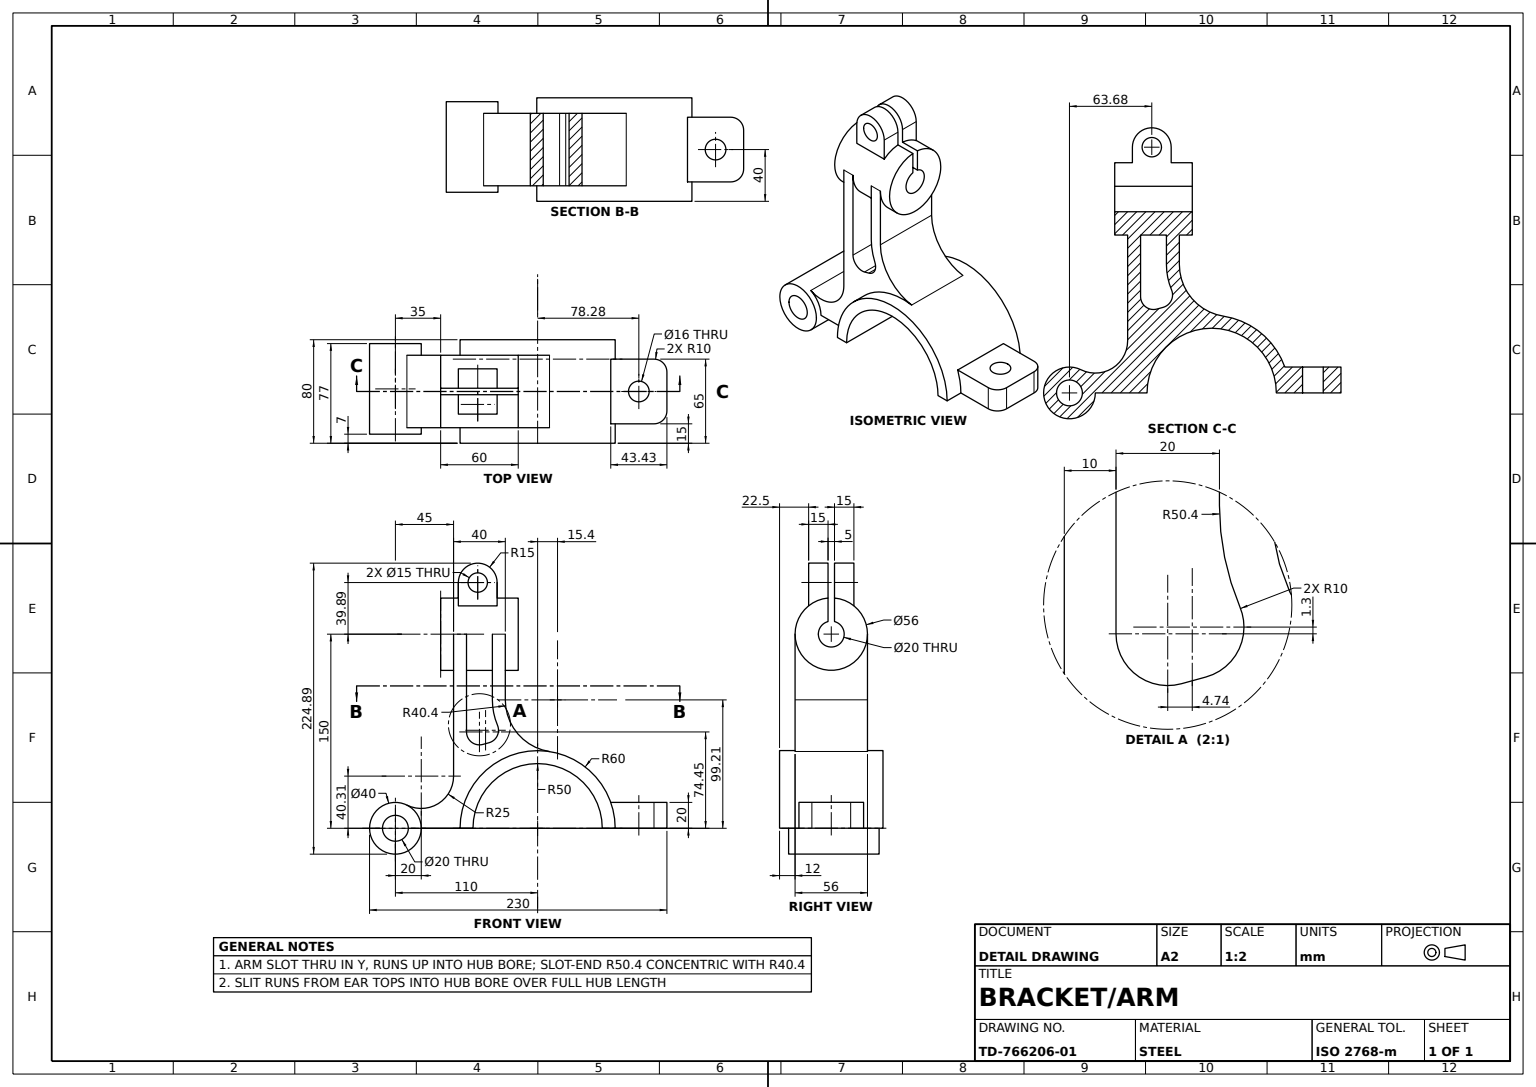
SolidWorks part; units mm, degrees
material "Plain Carbon Steel"
ref_plane "Front Plane" through (0, 0, 0) normal (0, 0, 1) x (1, 0, 0)
ref_plane "Top Plane" through (0, 0, 0) normal (0, 1, 0) x (1, 0, 0)
ref_plane "Right Plane" through (0, 0, 0) normal (1, 0, 0) x (0, 0, -1)
sketch "Base Block Sketch" plane through (0, 0, 0) normal (0, 0, 1) x (1, 0, 0)
  line L0 (-60, 0) -> (-50, 0)
  line L1 (50, 0) -> (60, 0)
  arc A0 (50, 0) -> (-50, 0) centre (0, 0) ccw
  arc A1 (60, 0) -> (-60, 0) centre (0, 0) ccw
  dimension "D1" = 60
  dimension "D2" = 50
extrude "Base Block" add sketch "Base Block Sketch" against normal mid plane 80
ref_plane "Plane1" through (0, 0, 28) normal (0, 0, 1) x (1, 0, 0)
sketch "Lower Hub Ø40 Sketch" plane through (0, 0, 28) normal (0, 0, 1) x (1, 0, 0)
  circle A0 centre (-110, 0) radius 20
  dimension "D1" = 40
  dimension "D2" = 110
extrude "Lower Hub Ø40" add sketch "Lower Hub Ø40 Sketch" along normal blind 5 and the other way blind 65 separate body
ref_plane "Plane2" through (-15, 0, 0) normal (1, 0, 0) x (0, 0, -1)
sketch "Upper Hub Ø56 Sketch" plane through (-15, 0, 0) normal (1, 0, 0) x (0, 0, -1)
  circle A0 centre (0, 150) radius 28
  dimension "D1" = 56
  dimension "D2" = 150
extrude "Upper Hub Ø56" add sketch "Upper Hub Ø56 Sketch" against normal blind 60 separate body
sketch "Web Arm Profile" plane through (0, 0, 0) normal (0, 0, 1) x (1, 0, 0)
  line L0 (-55, 150) -> (-55, 74.4461)
  line L2 (-65, 150) -> (-65, 40.3113)
  line L3 (-15, 150) -> (-25, 150)
  line L4 (-15, 122) -> (-15, 178) construction
  line L5 (-25, 150) -> (-25, 99.2112)
  line L6 (-15, 160) -> (-35, 160)
  line L7 (-35, 160) -> (-35, 99.2112)
  line L8 (-65, 150) -> (-25, 150)
  line L9 (-42.3554, 64.8021) -> (-37.6113, 66.103)
  line L10 (-60, 0) -> (-90, 0)
  line L11 (-55, 150) -> (-55, 40.3113) construction
  circle A0 centre (-110, 0) radius 20
  arc A1 (-101.1111, 17.9161) -> (-65, 40.3113) centre (-90, 40.3113) ccw
  arc A2 (9.2028, 59.29) -> (-60, 0) centre (0, 0) ccw
  arc A3 (-55, 74.4461) -> (-42.3554, 64.8021) centre (-45, 74.4461) ccw
  arc A5 (-25, 99.2112) -> (9.2028, 59.29) centre (15.3992, 99.2112) ccw
  arc A6 (-35, 99.2112) -> (-31.0414, 79.6318) centre (15.3992, 99.2112) ccw
  arc A7 (-35, 99.2112) -> (7.669, 49.4084) centre (15.3992, 99.2112) ccw construction
  arc A8 (-105.5556, 8.9581) -> (-55, 40.3113) centre (-90, 40.3113) ccw construction
  arc A9 (-37.6113, 66.103) -> (-31.0414, 79.6318) centre (-40.2559, 75.747) ccw
  dimension "D3" = 40
  dimension "D4" = 10
  dimension "D6" = 60
  dimension "D8" = 50.3992
  dimension "D10" = 10
  dimension "D7" = 25
  dimension "D12" = 10
  dimension "D1" = 10
  dimension "D2" = 65
  dimension "D5" = 10
  dimension "D9" = 57.8285
  dimension "D11" = 74.4461
extrude "Web Arm" add sketch "Web Arm Profile" against normal mid plane 56 contours A9 L9 A3 L0 L8 L2 A1 A0 L10 A2 A5 L5 L7 A6
sketch "Split Slot Sketch" plane through (-75, 0, 0) normal (-1, 0, 0) x (0, 0, 1)
  line L0 (0, 150) -> (2.5, 150)
  line L1 (2.5, 150) -> (2.5, 181.8317)
  line L2 (2.5, 181.8317) -> (-2.5, 181.8317)
  line L3 (-2.5, 181.8317) -> (-2.5, 150)
  line L4 (-2.5, 150) -> (0, 150)
  arc A0 (-2.5, 159.6825) -> (2.5, 159.6825) centre (0, 150) ccw
  circle M4 centre (0, 150) radius 28
  dimension "D1" = 31.8317
  dimension "D4" = 20
  dimension "D2" = 5
  dimension "D3" = 2.5
extrude "Split Slot" cut sketch "Split Slot Sketch" against normal blind 101 contours L3 L4 L0 L1 M4 | L3 A0 L1 L0 L4
sketch "Clamp Ear Sketch" plane through (0, 0, -2.5) normal (0, 0, 1) x (1, 0, 0)
  line L0 (-31.3234, 177.8882) -> (-31.3234, 149.8882)
  line L1 (-15, 177.8882) -> (-75, 177.8882) construction
  line L2 (-31.3234, 189.8882) -> (-31.3234, 177.8882)
  line L4 (-61.3234, 177.8882) -> (-61.3234, 189.8882)
  line L5 (-31.3234, 149.8882) -> (-61.3234, 150)
  line L6 (-65, 150) -> (-55, 150) construction
  line L7 (-61.3234, 150) -> (-61.3234, 177.8882)
  arc A0 (-31.3234, 189.8882) -> (-61.3234, 189.8882) centre (-46.3234, 189.8882) ccw
  dimension "D1" = 15
  dimension "D2" = 12
  dimension "D3" = 46.3234
  dimension "D4" = 27.9998
extrude "Clamp Ear" add sketch "Clamp Ear Sketch" against normal blind 15
mirror "Clamp Ear Mirror" about plane through (0, 0, 0) normal (0, 0, 1) of "Clamp Ear"
sketch "Upper Bore Ø20 Sketch" plane through (-15, 0, 0) normal (1, 0, 0) x (0, 0, -1)
  circle A0 centre (0, 150) radius 10
  dimension "D1" = 20
extrude "Upper Bore Ø20" cut sketch "Upper Bore Ø20 Sketch" against normal blind 89
sketch "Clamp Screw Hole Ø15 Sketch" plane through (0, 0, 17.5) normal (0, 0, 1) x (1, 0, 0)
  circle A0 centre (-46.3234, 189.8882) radius 7.5
  dimension "D1" = 15
extrude "Clamp Screw Hole Ø15" cut sketch "Clamp Screw Hole Ø15 Sketch" against normal blind 89
sketch "Lower Bore Ø20 Sketch" plane through (0, 0, 33) normal (0, 0, 1) x (1, 0, 0)
  circle A0 centre (-110, 0) radius 10
  dimension "D1" = 20
extrude "Lower Bore Ø20" cut sketch "Lower Bore Ø20 Sketch" against normal blind 89
sketch "Mounting Foot Sketch" plane through (0, 0, 0) normal (0, -1, 0) x (1, 0, 0)
  line L0 (50, 40) -> (60, 40) construction
  line L1 (100, 0) -> (100, 15)
  line L2 (90, 25) -> (50, 25)
  line L3 (50, -40) -> (50, 40) construction
  line L4 (50, 25) -> (50, -25)
  line L5 (50, -25) -> (90, -25)
  line L6 (100, -15) -> (100, 0)
  arc A0 (90, -25) -> (100, -15) centre (90, -15) ccw
  arc A1 (100, 15) -> (90, 25) centre (90, 15) ccw
  dimension "D1" = 10
  dimension "D2" = 50
  dimension "D3" = 50
  dimension "D4" = 25
  dimension "D5" = 15
extrude "Mounting Foot" add sketch "Mounting Foot Sketch" against normal blind 20
sketch "Foot Hole Ø16 Sketch" plane through (0, 20, 0) normal (0, 1, 0) x (1, 0, 0)
  circle A0 centre (78.2843, 0) radius 8
  dimension "D1" = 16
  dimension "D2" = 78.2843
extrude "Foot Hole Ø16" cut sketch "Foot Hole Ø16 Sketch" against normal blind 45
